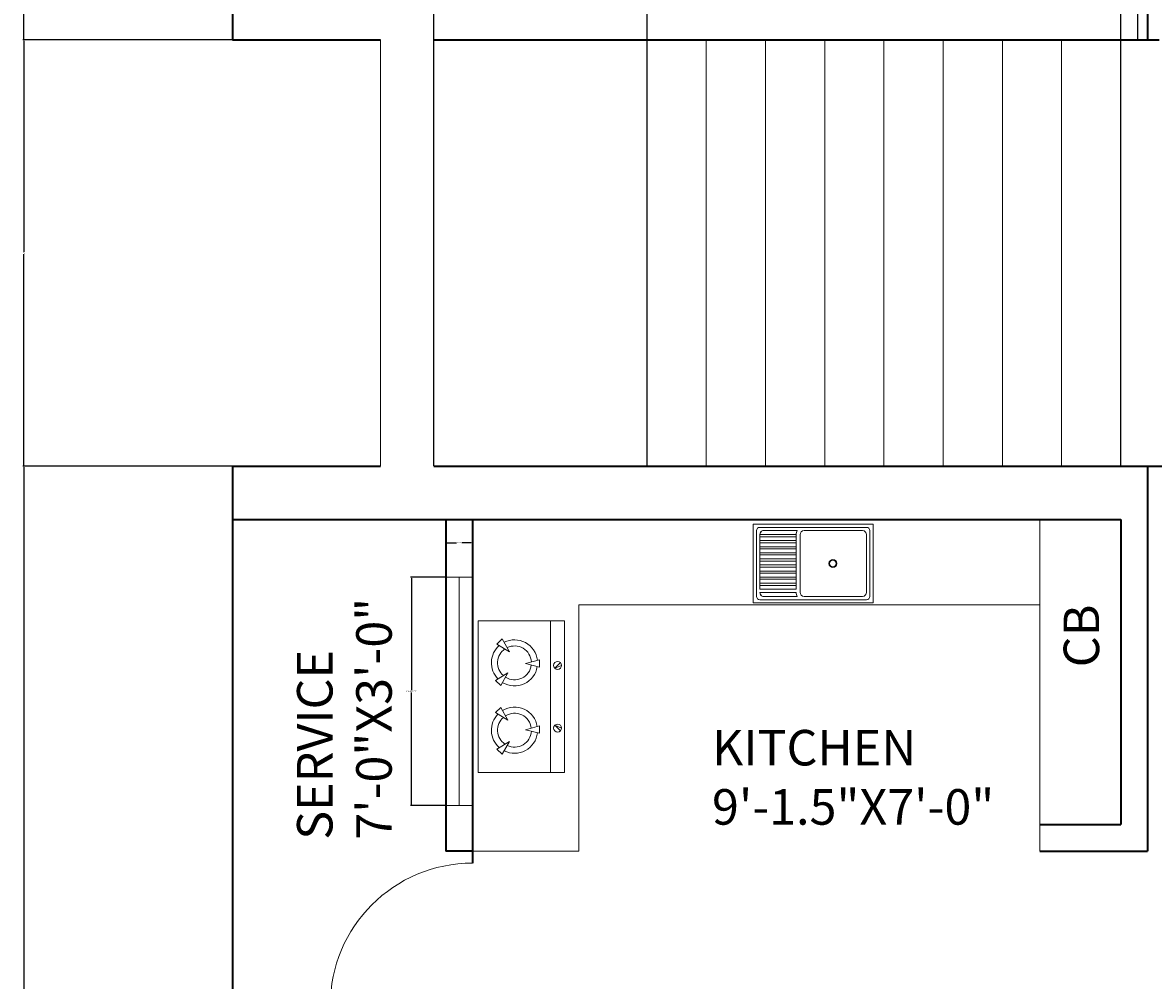
# Model space of a CAD drawing. Units: inches. Extents: x -59 to 444, y -680 to 63.
# Tile 3 of 9: x -59 to 132, y -431 to -270. Entities that reach past the tile are written whole.
import ezdxf

# ---------------------------------------------------------------- set-up
doc = ezdxf.new("R2010")
doc.units = ezdxf.units.IN
doc.header["$MEASUREMENT"] = 0
for name, color, linetype, lineweight in [('A-ANNO-DIMS', 2, 'Continuous', 18), ('A-ANNO-TEXT', 7, 'Continuous', 18), ('A-AREA-IDEN', 7, 'Continuous', 18), ('A-DOOR', 3, 'Continuous', 18), ('A-EQPM', 9, 'Continuous', 18), ('A-FLOR-CASE', 8, 'Continuous', 18), ('A-FLOR-FIXT', 9, 'Continuous', 18), ('A-FLOR-STRS', 7, 'Continuous', 18), ('A-GLAZ', 4, 'Continuous', 18), ('A-WALL', 7, 'Continuous', 35)]:
    doc.layers.add(name, color=color, linetype=linetype, lineweight=lineweight)
doc.styles.get("Standard").update_dxf_attribs({"font": 'arial.ttf'})
doc.dimstyles.get("Standard").update_dxf_attribs({"dimtxt": 0.18, "dimasz": 0.18, "dimexe": 0.18, "dimexo": 0.0625, "dimgap": 0.09, "dimtad": 0, "dimtih": 1, "dimtoh": 1, "dimdec": 0, "dimzin": 0, "dimdsep": 46, "dimlunit": 3, "dimtxsty": 'Standard', "dimcen": 0.09, "dimadec": 0, "dimazin": 0, "dimtfac": 1, "dimtdec": 0, "dimtofl": 0, "dimtmove": 0, "dimatfit": 3, "dimfxl": 1, "dimtolj": 1, "dimtzin": 0, "dimarcsym": 0})

# ---------------------------------------------------------------- blocks, each defined once
blk = doc.blocks.new('М12 540х820')
for p, q in [((0, 540), (-820, 540)), ((-820, 540), (-820, 0)), ((-797.5, 495), (-797.5, 45)), ((-45, 517.5), (-775, 517.5)), ((-775, 468), (-775, 72)), ((-347.5, 495), (-748, 495)), ((-320.5, 468), (-320.5, 72)), ((-301.7, 495), (-64.8, 495)), ((-293.7, 468), (-293.7, 472.5)), ((-293.7, 468), (-45, 468)), ((-45, 469.5), (-45, 468)), ((-22.5, 45), (-22.5, 495)), ((0, 0), (0, 540)), ((-293.7, 446.6), (-45, 446.6)), ((-293.7, 419.6), (-293.7, 446.6)), ((-293.7, 419.6), (-45, 419.6)), ((-293.7, 405), (-45, 405)), ((-293.7, 378), (-293.7, 405)), ((-45, 419.6), (-45, 446.6)), ((-45, 378), (-45, 405)), ((-293.7, 378), (-45, 378)), ((-293.7, 336.4), (-293.7, 363.4)), ((-293.7, 363.4), (-45, 363.4)), ((-293.7, 336.4), (-45, 336.4)), ((-293.7, 294.7), (-293.7, 321.7)), ((-293.7, 321.7), (-45, 321.7)), ((-45, 336.4), (-45, 363.4)), ((-45, 294.7), (-45, 321.7)), ((-293.7, 294.7), (-45, 294.7)), ((-293.7, 253.1), (-293.7, 280.1)), ((-293.7, 280.1), (-45, 280.1)), ((-293.7, 253.1), (-45, 253.1)), ((-293.7, 211.5), (-293.7, 238.5)), ((-293.7, 238.5), (-45, 238.5)), ((-45, 253.1), (-45, 280.1)), ((-45, 211.5), (-45, 238.5)), ((-293.7, 211.5), (-45, 211.5)), ((-293.7, 169.9), (-293.7, 196.9)), ((-293.7, 196.9), (-45, 196.9)), ((-293.7, 169.9), (-45, 169.9)), ((-293.7, 128.2), (-293.7, 155.2)), ((-293.7, 155.2), (-45, 155.2)), ((-45, 169.9), (-45, 196.9)), ((-45, 128.2), (-45, 155.2)), ((-293.7, 128.2), (-45, 128.2)), ((-293.7, 113.6), (-45, 113.6)), ((-293.7, 86.6), (-293.7, 113.6)), ((-293.7, 86.6), (-45, 86.6)), ((-45, 86.6), (-45, 113.6)), ((-820, 0), (0, 0)), ((-775, 22.5), (-45, 22.5)), ((-748, 45), (-347.5, 45)), ((-301.7, 45), (-64.8, 45)), ((-293.7, 72), (-45, 72)), ((-45, 70.5), (-45, 72))]:
    blk.add_line(p, q)
at = {"ltscale": 0.06}
for p, q in [((-820, 0), (-820, 540)), ((-820, 540), (0, 540)), ((0, 540), (0, 536.9)), ((0, 536.9), (0, 0)), ((-293.7, 446.6), (-45, 446.6)), ((-293.7, 405), (-293.7, 446.6)), ((-293.7, 363.4), (-293.7, 405)), ((-45, 446.6), (-45, 419.6)), ((-45, 419.6), (-45, 378)), ((-293.7, 321.7), (-293.7, 363.4)), ((-293.7, 280.1), (-293.7, 321.7)), ((-45, 378), (-45, 336.4)), ((-45, 336.4), (-45, 294.7)), ((-293.7, 238.5), (-293.7, 280.1)), ((-293.7, 196.9), (-293.7, 238.5)), ((-45, 294.7), (-45, 253.1)), ((-45, 253.1), (-45, 211.5)), ((-293.7, 155.2), (-293.7, 196.9)), ((-293.7, 113.6), (-293.7, 155.2)), ((-45, 211.5), (-45, 169.9)), ((-45, 169.9), (-45, 128.2)), ((-293.7, 72), (-293.7, 113.6)), ((-45, 128.2), (-45, 86.6)), ((-45, 86.6), (-45, 72)), ((0, 0), (-820, 0)), ((-45, 72), (-293.7, 72))]:
    blk.add_line(p, q, dxfattribs=at)
at = {"extrusion": (0, 0, -1)}
for centre, major_axis, start_param, end_param in [((-775, 495), (-15.9, 15.9), -0.785398, 0.785398), ((-775, 495), (-15.9, 15.9), -0.785398, 0.785398), ((-748, 468), (-19.1, -19.1), 0.785398, 2.356194), ((-748, 468), (-19.1, -19.1), 0.785398, 2.356194), ((-347.5, 468), (-19.1, 19.1), 0.785398, 2.356194), ((-347.5, 468), (-19.1, 19.1), 0.785398, 2.356194), ((-343.2, 468), (-35, 35), 1.779263, 2.356194), ((-343.2, 468), (-35, 35), 1.779263, 2.356192), ((-343.2, 468), (-35, 35), 2.356192, 2.356194), ((-72.3, 468.8), (-19.3, 19.3), 1.0328, 2.38382), ((-72.3, 468.8), (-19.3, 19.3), 1.0328, 1.064673), ((-72.3, 468.8), (-19.3, 19.3), 1.064673, 2.328569), ((-45, 495), (-15.9, -15.9), 2.356194, 3.926991), ((-45, 495), (-15.9, -15.9), 2.356194, 3.926991), ((-72.3, 468.8), (-19.3, 19.3), 2.328569, 2.38382), ((-545.5, 270), (-19.1, -19.1), 3.926991, 10.210176), ((-545.5, 270), (-19.1, -19.1), 3.926991, 10.210176), ((-545.5, 270), (-15.9, -15.9), 3.926991, 10.210176), ((-545.5, 270), (-15.9, -15.9), 3.926991, 10.210176), ((-775, 45), (-15.9, -15.9), 5.497787, 7.068583), ((-775, 45), (-15.9, -15.9), 5.497787, 7.068583), ((-748, 72), (-19.1, 19.1), 3.926991, 5.497787), ((-748, 72), (-19.1, 19.1), 3.926991, 5.497787), ((-347.5, 72), (-19.1, -19.1), 3.926991, 5.497787), ((-347.5, 72), (-19.1, -19.1), 3.926991, 5.497787), ((-343.2, 72), (-35, -35), 3.926991, 4.503922), ((-343.2, 72), (-35, -35), 3.926991, 4.503922), ((-72.3, 71.2), (-19.3, -19.3), 3.899365, 5.250385), ((-72.3, 71.2), (-19.3, -19.3), 5.218512, 5.250385), ((-72.3, 71.2), (-19.3, -19.3), 3.954617, 5.218512), ((-72.3, 71.2), (-19.3, -19.3), 3.899365, 3.954617), ((-45, 45), (-15.9, 15.9), 2.356194, 3.926991), ((-45, 45), (-15.9, 15.9), 2.356194, 3.926991)]:
    blk.add_ellipse(centre, major_axis=major_axis, ratio=1, start_param=start_param, end_param=end_param, dxfattribs=at)
blk = doc.blocks.new('WIN-SERVICE')
for p, q in [((0, 38.53), (0, 0)), ((4.5, 38.53), (0, 38.53)), ((2.25, 38.53), (2.25, 0)), ((4.5, 38.53), (4.5, 0)), ((0, 0), (4.5, 0))]:
    blk.add_line(p, q)
blk = doc.blocks.new('DOOR-SWING-24')
blk.add_line((24, 0), (0, 0))
blk.add_arc((24, 0), 24, 90, 180)
blk = doc.blocks.new('*D17')
at = {"layer": 'A-ANNO-DIMS', "color": 0, "lineweight": -2, "transparency": 16777216}
for p, q in [((133.17, -248.44), (129.45, -248.44)), ((129.63, -248.62), (129.63, -260.25)), ((129.63, -272.26), (129.63, -260.62)), ((133.17, -272.44), (129.45, -272.44))]:
    blk.add_line(p, q, dxfattribs=at)
at = {"layer": 'A-ANNO-DIMS', "color": 0, "transparency": 16777216}
for points in [[(129.6, -248.62), (129.66, -248.62), (129.63, -248.44)], [(129.6, -272.26), (129.66, -272.26), (129.63, -272.44)]]:
    blk.add_solid(points, dxfattribs=at)
at = {"layer": 'Defpoints', "color": 0, "transparency": 16777216}
for p in [(133.23, -248.44), (129.63, -272.44), (133.23, -272.44)]:
    blk.add_point(p, dxfattribs=at)
at = {"layer": 'A-ANNO-DIMS', "color": 0, "transparency": 16777216, "insert": (129.63, -260.44), "char_height": 0.18, "attachment_point": 5}
blk.add_mtext('\\A1;24 TYP.', dxfattribs=at)
blk = doc.blocks.new('*D26')
at = {"layer": 'A-ANNO-DIMS', "color": 0, "lineweight": -2, "transparency": 16777216}
for p, q in [((12.67, -363.17), (6.77, -363.17)), ((6.95, -363.35), (6.95, -382.25)), ((6.95, -401.52), (6.95, -382.62)), ((12.67, -401.7), (6.77, -401.7))]:
    blk.add_line(p, q, dxfattribs=at)
at = {"layer": 'A-ANNO-DIMS', "color": 0, "transparency": 16777216}
for points in [[(6.92, -363.35), (6.98, -363.35), (6.95, -363.17)], [(6.92, -401.52), (6.98, -401.52), (6.95, -401.7)]]:
    blk.add_solid(points, dxfattribs=at)
at = {"layer": 'Defpoints', "color": 0, "transparency": 16777216}
for p in [(6.95, -363.17), (12.73, -363.17), (12.73, -401.7)]:
    blk.add_point(p, dxfattribs=at)
at = {"layer": 'A-ANNO-DIMS', "color": 0, "transparency": 16777216, "insert": (6.95, -382.44), "char_height": 0.18, "attachment_point": 5}
blk.add_mtext('\\A1;WINDOW 39 TYP.', dxfattribs=at)
blk = doc.blocks.new('*D27')
at = {"layer": 'A-ANNO-DIMS', "color": 0, "lineweight": -2, "transparency": 16777216}
for p, q in [((12.73, -363.11), (12.73, -357.21)), ((12.91, -357.39), (14.52, -357.39)), ((17.05, -357.39), (15.44, -357.39)), ((17.23, -363.11), (17.23, -357.21))]:
    blk.add_line(p, q, dxfattribs=at)
at = {"layer": 'A-ANNO-DIMS', "color": 0, "transparency": 16777216}
for points in [[(12.91, -357.36), (12.91, -357.42), (12.73, -357.39)], [(17.05, -357.36), (17.05, -357.42), (17.23, -357.39)]]:
    blk.add_solid(points, dxfattribs=at)
at = {"layer": 'Defpoints', "color": 0, "transparency": 16777216}
for p in [(17.23, -357.39), (12.73, -363.17), (17.23, -363.17)]:
    blk.add_point(p, dxfattribs=at)
at = {"layer": 'A-ANNO-DIMS', "color": 0, "transparency": 16777216, "insert": (14.98, -357.39), "char_height": 0.18, "attachment_point": 5}
blk.add_mtext('\\A1;5 TYP.', dxfattribs=at)
blk = doc.blocks.new('*D48')
at = {"layer": 'A-ANNO-DIMS', "color": 0, "lineweight": -2, "transparency": 16777216}
for p, q in [((-23.33, 15.56), (-58.7, 15.56)), ((-58.52, 15.38), (-58.52, -128.25)), ((-58.52, -272.26), (-58.52, -128.62)), ((-23.33, -272.44), (-58.7, -272.44))]:
    blk.add_line(p, q, dxfattribs=at)
at = {"layer": 'A-ANNO-DIMS', "color": 0, "transparency": 16777216}
for points in [[(-58.55, 15.38), (-58.49, 15.38), (-58.52, 15.56)], [(-58.55, -272.26), (-58.49, -272.26), (-58.52, -272.44)]]:
    blk.add_solid(points, dxfattribs=at)
at = {"layer": 'Defpoints', "color": 0, "transparency": 16777216}
for p in [(-23.27, 15.56), (-58.52, -272.44), (-23.27, -272.44)]:
    blk.add_point(p, dxfattribs=at)
at = {"layer": 'A-ANNO-DIMS', "color": 0, "transparency": 16777216, "insert": (-58.52, -128.44), "char_height": 0.18, "attachment_point": 5}
blk.add_mtext('\\A1;288', dxfattribs=at)
blk = doc.blocks.new('*D49')
at = {"layer": 'A-ANNO-DIMS', "color": 0, "lineweight": -2, "transparency": 16777216}
for p, q in [((-23.33, -272.44), (-58.7, -272.44)), ((-58.52, -272.62), (-58.52, -308.25)), ((-58.52, -344.26), (-58.52, -308.62)), ((-23.33, -344.44), (-58.7, -344.44))]:
    blk.add_line(p, q, dxfattribs=at)
at = {"layer": 'A-ANNO-DIMS', "color": 0, "transparency": 16777216}
for points in [[(-58.55, -272.62), (-58.49, -272.62), (-58.52, -272.44)], [(-58.55, -344.26), (-58.49, -344.26), (-58.52, -344.44)]]:
    blk.add_solid(points, dxfattribs=at)
at = {"layer": 'Defpoints', "color": 0, "transparency": 16777216}
for p in [(-23.27, -272.44), (-58.52, -344.44), (-23.27, -344.44)]:
    blk.add_point(p, dxfattribs=at)
at = {"layer": 'A-ANNO-DIMS', "color": 0, "transparency": 16777216, "insert": (-58.52, -308.44), "char_height": 0.18, "attachment_point": 5}
blk.add_mtext('\\A1;72', dxfattribs=at)
blk = doc.blocks.new('*D50')
at = {"layer": 'A-ANNO-DIMS', "color": 0, "lineweight": -2, "transparency": 16777216}
for p, q in [((-23.33, -344.44), (-58.7, -344.44)), ((-58.52, -344.62), (-58.52, -488.25)), ((-58.52, -632.26), (-58.52, -488.62)), ((-23.33, -632.44), (-58.7, -632.44))]:
    blk.add_line(p, q, dxfattribs=at)
at = {"layer": 'A-ANNO-DIMS', "color": 0, "transparency": 16777216}
for points in [[(-58.55, -344.62), (-58.49, -344.62), (-58.52, -344.44)], [(-58.55, -632.26), (-58.49, -632.26), (-58.52, -632.44)]]:
    blk.add_solid(points, dxfattribs=at)
at = {"layer": 'Defpoints', "color": 0, "transparency": 16777216}
for p in [(-23.27, -344.44), (-58.52, -632.44), (-23.27, -632.44)]:
    blk.add_point(p, dxfattribs=at)
at = {"layer": 'A-ANNO-DIMS', "color": 0, "transparency": 16777216, "insert": (-58.52, -488.44), "char_height": 0.18, "attachment_point": 5}
blk.add_mtext('\\A1;288', dxfattribs=at)
blk = doc.blocks.new('*D54')
at = {"layer": 'A-ANNO-DIMS', "color": 0, "lineweight": -2, "transparency": 16777216}
for p, q in [((10.73, -344.37), (10.73, 62.74)), ((10.91, 62.56), (28.51, 62.56)), ((46.55, 62.56), (28.95, 62.56)), ((46.73, -344.37), (46.73, 62.74))]:
    blk.add_line(p, q, dxfattribs=at)
at = {"layer": 'A-ANNO-DIMS', "color": 0, "transparency": 16777216}
for points in [[(10.91, 62.59), (10.91, 62.53), (10.73, 62.56)], [(46.55, 62.59), (46.55, 62.53), (46.73, 62.56)]]:
    blk.add_solid(points, dxfattribs=at)
at = {"layer": 'Defpoints', "color": 0, "transparency": 16777216}
for p in [(46.73, 62.56), (10.73, -344.44), (46.73, -344.44)]:
    blk.add_point(p, dxfattribs=at)
at = {"layer": 'A-ANNO-DIMS', "color": 0, "transparency": 16777216, "insert": (28.73, 62.56), "char_height": 0.18, "attachment_point": 5}
blk.add_mtext('\\A1;36', dxfattribs=at)
blk = doc.blocks.new('*D55')
at = {"layer": 'A-ANNO-DIMS', "color": 0, "lineweight": -2, "transparency": 16777216}
for p, q in [((46.73, -344.37), (46.73, 62.74)), ((46.91, 62.56), (86.51, 62.56)), ((126.55, 62.56), (86.95, 62.56)), ((126.73, -344.37), (126.73, 62.74))]:
    blk.add_line(p, q, dxfattribs=at)
at = {"layer": 'A-ANNO-DIMS', "color": 0, "transparency": 16777216}
for points in [[(46.91, 62.59), (46.91, 62.53), (46.73, 62.56)], [(126.55, 62.59), (126.55, 62.53), (126.73, 62.56)]]:
    blk.add_solid(points, dxfattribs=at)
at = {"layer": 'Defpoints', "color": 0, "transparency": 16777216}
for p in [(126.73, 62.56), (46.73, -344.44), (126.73, -344.44)]:
    blk.add_point(p, dxfattribs=at)
at = {"layer": 'A-ANNO-DIMS', "color": 0, "transparency": 16777216, "insert": (86.73, 62.56), "char_height": 0.18, "attachment_point": 5}
blk.add_mtext('\\A1;80', dxfattribs=at)
blk = doc.blocks.new('*D56')
at = {"layer": 'A-ANNO-DIMS', "color": 0, "lineweight": -2, "transparency": 16777216}
for p, q in [((126.73, -344.37), (126.73, 62.74)), ((126.91, 62.56), (158.65, 62.56)), ((191.05, 62.56), (159.3, 62.56)), ((191.23, -344.37), (191.23, 62.74))]:
    blk.add_line(p, q, dxfattribs=at)
at = {"layer": 'A-ANNO-DIMS', "color": 0, "transparency": 16777216}
for points in [[(126.91, 62.59), (126.91, 62.53), (126.73, 62.56)], [(191.05, 62.59), (191.05, 62.53), (191.23, 62.56)]]:
    blk.add_solid(points, dxfattribs=at)
at = {"layer": 'Defpoints', "color": 0, "transparency": 16777216}
for p in [(191.23, 62.56), (126.73, -344.44), (191.23, -344.44)]:
    blk.add_point(p, dxfattribs=at)
at = {"layer": 'A-ANNO-DIMS', "color": 0, "transparency": 16777216, "insert": (158.98, 62.56), "char_height": 0.18, "attachment_point": 5}
blk.add_mtext('\\A1;64.5', dxfattribs=at)

msp = doc.modelspace()

# ---------------------------------------------------------------- linework, layer by layer
at = {"layer": 'A-EQPM'}
for p, q in [((30.43, -370.56), (30.43, -396.15)), ((21.35, -374.45), (22.26, -373.57)), ((22.26, -373.57), (23.47, -375.75)), ((23.47, -375.75), (21.35, -374.45)), ((26.19, -377.72), (28.59, -377.12)), ((28.59, -378.38), (26.19, -377.72)), ((28.59, -377.12), (28.59, -378.38)), ((21.12, -380.62), (23.24, -379.31)), ((23.24, -379.31), (22.05, -381.48)), ((22.05, -381.48), (21.12, -380.62)), ((22.05, -385.16), (21.12, -386.02)), ((23.24, -387.33), (22.05, -385.16)), ((21.12, -386.02), (23.24, -387.33)), ((28.59, -388.26), (26.19, -388.92)), ((26.19, -388.92), (28.59, -389.53)), ((28.59, -389.53), (28.59, -388.26)), ((23.47, -390.89), (21.35, -392.19)), ((22.26, -393.07), (23.47, -390.89)), ((21.35, -392.19), (22.26, -393.07))]:
    msp.add_line(p, q, dxfattribs=at)
at = {"layer": 'A-EQPM', "ltscale": 20}
for p, q in [((31.15, -378.54), (32.1, -377.59)), ((32.29, -378.06), (31.15, -378.54)), ((31.15, -388.16), (32.1, -389.12)), ((32.29, -388.64), (31.15, -388.16))]:
    msp.add_line(p, q, dxfattribs=at)
at = {"layer": 'A-EQPM'}
msp.add_lwpolyline([(18.19, -396.15), (18.19, -370.56), (32.81, -370.56), (32.81, -396.15)], close=True, dxfattribs=at)
at = {"layer": 'A-EQPM', "ltscale": 20}
for centre in [(31.62, -378.07), (31.62, -388.64)]:
    msp.add_circle(centre, 0.673, dxfattribs=at)
at = {"layer": 'A-EQPM'}
for centre, radius, start, end in [((24.34, -377.64), 3.9, 6.4005, 116.769), ((24.34, -377.64), 3.9, 131.2225, 224.1627), ((24.34, -377.64), 2.86, 124.5561, 228.8027), ((24.34, -377.64), 2.86, 3.5753, 115.9207), ((24.34, -377.64), 2.86, 237.9778, 353.02), ((24.34, -377.64), 3.9, 238.853, 350.7562), ((24.34, -389), 3.9, 9.2438, 121.147), ((24.34, -389), 3.9, 135.8373, 228.7775), ((24.34, -389), 2.86, 131.1973, 235.4439), ((24.34, -389), 2.86, 6.98, 122.0222), ((24.34, -389), 3.9, 243.231, 353.5995), ((24.34, -389), 2.86, 244.0793, 356.4247)]:
    msp.add_arc(centre, radius, start, end, dxfattribs=at)
at = {"layer": 'A-FLOR-CASE'}
for p, q in [((113.04, -409.44), (113.04, -353.44)), ((113.04, -367.85), (35.21, -367.85)), ((35.21, -367.85), (35.21, -409.44)), ((17.23, -409.44), (35.21, -409.44))]:
    msp.add_line(p, q, dxfattribs=at)
at = {"layer": 'A-FLOR-STRS'}
for p, q in [((1.73, -344.44), (1.73, -272.44)), ((10.73, -344.44), (10.73, -272.44)), ((46.73, -344.44), (46.73, -272.44)), ((56.73, -344.44), (56.73, -272.44)), ((66.73, -344.44), (66.73, -272.44)), ((76.73, -344.44), (76.73, -272.44)), ((86.73, -344.44), (86.73, -272.44)), ((96.73, -344.44), (96.73, -272.44)), ((106.73, -344.44), (106.73, -272.44)), ((116.73, -344.44), (116.73, -272.44)), ((126.73, -344.44), (126.73, -272.44))]:
    msp.add_line(p, q, dxfattribs=at)
at = {"layer": 'A-WALL'}
for p, q in [((-23.27, 15.56), (-23.27, -272.44)), ((131.23, -160.44), (131.23, -272.44)), ((-23.27, -272.44), (1.73, -272.44)), ((10.73, -272.44), (133.23, -272.44)), ((-23.27, -344.44), (1.73, -344.44)), ((-23.27, -344.44), (-23.27, -632.44)), ((10.73, -344.44), (191.23, -344.44)), ((131.23, -344.44), (131.23, -409.44)), ((-23.27, -353.44), (126.73, -353.44)), ((12.73, -353.44), (12.73, -409.44)), ((17.23, -353.44), (17.23, -411.44)), ((126.73, -353.44), (126.73, -404.94)), ((113.04, -404.94), (126.73, -404.94)), ((17.23, -409.44), (12.73, -409.44)), ((113.04, -409.44), (131.23, -409.44))]:
    msp.add_line(p, q, dxfattribs=at)

# ---------------------------------------------------------------- block references
at = {"layer": 'A-DOOR'}
msp.add_blockref('DOOR-SWING-24', (-6.77, -435.44), dxfattribs=at)
at = {"layer": 'A-FLOR-FIXT', "xscale": 0.0246684035300764, "yscale": 0.0246684035300764, "zscale": 0.0246684035300764, "rotation": 180}
msp.add_blockref('М12 540х820', (64.66, -354.2), dxfattribs=at)
at = {"layer": 'A-GLAZ'}
msp.add_blockref('WIN-SERVICE', (12.73, -401.7), dxfattribs=at)

# ---------------------------------------------------------------- texts
at = {"layer": 'A-ANNO-TEXT', "insert": (117.07, -378.38), "char_height": 6, "attachment_point": 1, "rotation": 90}
msp.add_mtext('CB', dxfattribs=at)
at = {"layer": 'A-AREA-IDEN', "insert": (-12.39, -407.5), "char_height": 6, "attachment_point": 1, "rotation": 90}
msp.add_mtext('SERVICE\\P7\'-0"X3\'-0"', dxfattribs=at)
at = {"layer": 'A-AREA-IDEN', "insert": (57.69, -388.95), "char_height": 6, "attachment_point": 1}
msp.add_mtext_dynamic_manual_height_columns('KITCHEN\\P9\'-1.5"X7\'-0"', width=6, gutter_width=1, heights=[0], dxfattribs=at)

# ---------------------------------------------------------------- dimensions: what is measured, and where the dimension line sits
at = {"layer": 'A-ANNO-DIMS'}
for base, p1, p2, override, picture, middle in [((46.73, 62.56), (10.73, -344.44), (46.73, -344.44), {"dimdec": 0, "dimlfac": 1, "dimrnd": 0, "dimzin": 0, "dimdsep": 46, "dimlunit": 2}, '*D54', (28.73, 62.56)), ((126.73, 62.56), (46.73, -344.44), (126.73, -344.44), {"dimdec": 0, "dimlfac": 1, "dimrnd": 0, "dimzin": 0, "dimdsep": 46, "dimlunit": 2}, '*D55', (86.73, 62.56)), ((191.23, 62.56), (126.73, -344.44), (191.23, -344.44), {"dimdec": 1, "dimlfac": 1, "dimrnd": 0, "dimzin": 0, "dimdsep": 46, "dimlunit": 2}, '*D56', (158.98, 62.56))]:
    dim = msp.add_linear_dim(base=base, p1=p1, p2=p2, dimstyle='Standard', override=override, dxfattribs=at)
    dim.commit()
    dim.dimension.update_dxf_attribs({"geometry": picture, "text_midpoint": middle})
for base, p1, p2, picture, middle in [((-58.52, -272.44), (-23.27, 15.56), (-23.27, -272.44), '*D48', (-58.52, -128.44)), ((-58.52, -344.44), (-23.27, -272.44), (-23.27, -344.44), '*D49', (-58.52, -308.44)), ((-58.52, -632.44), (-23.27, -344.44), (-23.27, -632.44), '*D50', (-58.52, -488.44))]:
    dim = msp.add_linear_dim(base=base, p1=p1, p2=p2, angle=90, dimstyle='Standard', override={"dimdec": 0, "dimlfac": 1, "dimrnd": 0, "dimzin": 0, "dimdsep": 46, "dimlunit": 2}, dxfattribs=at)
    dim.commit()
    dim.dimension.update_dxf_attribs({"geometry": picture, "text_midpoint": middle})
for base, p1, p2, angle, text, picture, middle in [((129.63, -272.44), (133.23, -248.44), (133.23, -272.44), 270, '<> TYP.', '*D17', (129.63, -260.44)), ((6.95, -363.17), (12.73, -401.7), (12.73, -363.17), 90, 'WINDOW <> TYP.', '*D26', (6.95, -382.44))]:
    dim = msp.add_linear_dim(base=base, p1=p1, p2=p2, angle=angle, text=text, dimstyle='Standard', override={"dimdec": 0, "dimlfac": 1, "dimrnd": 0, "dimzin": 0, "dimdsep": 46, "dimlunit": 2}, dxfattribs=at)
    dim.commit()
    dim.dimension.update_dxf_attribs({"geometry": picture, "text_midpoint": middle})
dim = msp.add_linear_dim(base=(17.2298001, -357.39194777), p1=(12.7298001, -363.17118172), p2=(17.2298001, -363.17118172), text='<> TYP.', dimstyle='Standard', override={"dimdec": 0, "dimlfac": 1, "dimrnd": 0, "dimzin": 0, "dimdsep": 46, "dimlunit": 2}, dxfattribs=at)
dim.commit()
dim.dimension.update_dxf_attribs({"geometry": '*D27', "text_midpoint": (14.9798001, -357.39194777)})

doc.saveas('drawing.dxf')
